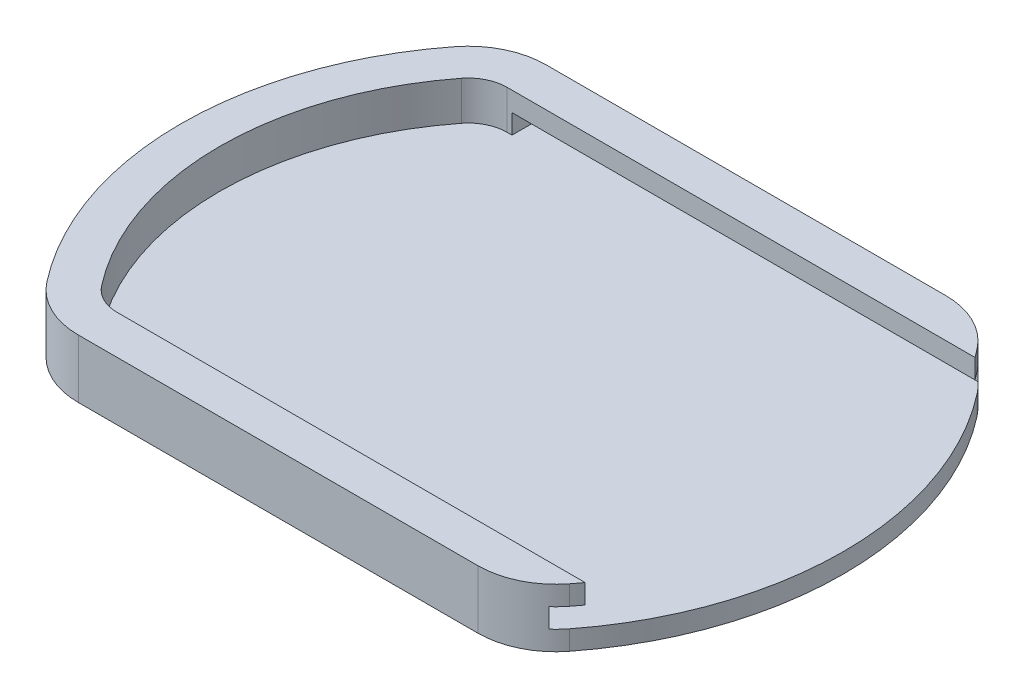
ISO-10303-21;
HEADER;
FILE_DESCRIPTION(('STEP AP214'),'2;1');
FILE_NAME('part.step','',(''),(''),'','','');
FILE_SCHEMA(('AUTOMOTIVE_DESIGN { 1 0 10303 214 1 1 1 1 }'));
ENDSEC;
DATA;
#1=APPLICATION_CONTEXT('core data for automotive mechanical design processes');
#2=APPLICATION_PROTOCOL_DEFINITION('international standard','automotive_design',2000,#1);
#3=PRODUCT_CONTEXT('',#1,'mechanical');
#4=PRODUCT('Part','Part','',(#3));
#5=PRODUCT_RELATED_PRODUCT_CATEGORY('part','',(#4));
#6=PRODUCT_DEFINITION_FORMATION('','',#4);
#7=PRODUCT_DEFINITION_CONTEXT('part definition',#1,'design');
#8=PRODUCT_DEFINITION('design','',#6,#7);
#9=PRODUCT_DEFINITION_SHAPE('','',#8);
#10=(LENGTH_UNIT() NAMED_UNIT(*) SI_UNIT(.MILLI.,.METRE.));
#11=(NAMED_UNIT(*) PLANE_ANGLE_UNIT() SI_UNIT($,.RADIAN.));
#12=(NAMED_UNIT(*) SI_UNIT($,.STERADIAN.) SOLID_ANGLE_UNIT());
#13=UNCERTAINTY_MEASURE_WITH_UNIT(LENGTH_MEASURE(1.E-05),#10,'distance_accuracy_value','');
#14=(GEOMETRIC_REPRESENTATION_CONTEXT(3) GLOBAL_UNCERTAINTY_ASSIGNED_CONTEXT((#13)) GLOBAL_UNIT_ASSIGNED_CONTEXT((#10,
#11,#12)) REPRESENTATION_CONTEXT('',''));
#15=CARTESIAN_POINT('',(0.,0.,0.));
#16=DIRECTION('',(0.,0.,1.));
#17=DIRECTION('',(1.,0.,0.));
#18=AXIS2_PLACEMENT_3D('',#15,#16,#17);
#19=CARTESIAN_POINT('',(0.,1.,0.));
#20=DIRECTION('',(0.,-1.,0.));
#21=DIRECTION('',(0.,0.,-1.));
#22=AXIS2_PLACEMENT_3D('',#19,#20,#21);
#23=CYLINDRICAL_SURFACE('',#22,17.);
#24=CARTESIAN_POINT('',(0.,2.,0.));
#25=DIRECTION('',(0.,1.,0.));
#26=DIRECTION('',(0.,0.,1.));
#27=AXIS2_PLACEMENT_3D('',#24,#25,#26);
#28=CIRCLE('',#27,17.);
#29=CARTESIAN_POINT('',(13.3998586939472,2.,-10.4615384615385));
#30=VERTEX_POINT('',#29);
#31=CARTESIAN_POINT('',(13.7477270848675,2.,-10.));
#32=VERTEX_POINT('',#31);
#33=EDGE_CURVE('E415',#30,#32,#28,.F.);
#34=ORIENTED_EDGE('',*,*,#33,.F.);
#35=DIRECTION('',(0.,-1.,0.));
#36=VECTOR('',#35,1.);
#37=CARTESIAN_POINT('',(13.3998586939472,1.,-10.4615384615385));
#38=LINE('',#37,#36);
#39=CARTESIAN_POINT('',(13.3998586939472,3.,-10.4615384615385));
#40=VERTEX_POINT('',#39);
#41=EDGE_CURVE('E283',#40,#30,#38,.T.);
#42=ORIENTED_EDGE('',*,*,#41,.F.);
#43=CARTESIAN_POINT('',(0.,3.,0.));
#44=DIRECTION('',(0.,1.,0.));
#45=DIRECTION('',(0.,0.,1.));
#46=AXIS2_PLACEMENT_3D('',#43,#44,#45);
#47=CIRCLE('',#46,17.);
#48=CARTESIAN_POINT('',(13.7477270848675,3.,-10.));
#49=VERTEX_POINT('',#48);
#50=EDGE_CURVE('E318',#49,#40,#47,.T.);
#51=ORIENTED_EDGE('',*,*,#50,.F.);
#52=DIRECTION('',(0.,-1.,0.));
#53=VECTOR('',#52,1.);
#54=CARTESIAN_POINT('',(13.7477270848675,3.,-10.));
#55=LINE('',#54,#53);
#56=EDGE_CURVE('E235',#49,#32,#55,.T.);
#57=ORIENTED_EDGE('',*,*,#56,.T.);
#58=EDGE_LOOP('',(#34,#42,#51,#57));
#59=FACE_BOUND('',#58,.T.);
#60=ADVANCED_FACE('F41',(#59),#23,.T.);
#61=CARTESIAN_POINT('',(13.3998586939472,1.,-10.4615384615385));
#62=VERTEX_POINT('',#61);
#63=CARTESIAN_POINT('',(13.3998586939472,0.,-10.4615384615385));
#64=VERTEX_POINT('',#63);
#65=EDGE_CURVE('E281',#62,#64,#38,.T.);
#66=ORIENTED_EDGE('',*,*,#65,.F.);
#67=CARTESIAN_POINT('',(0.,1.,0.));
#68=DIRECTION('',(0.,1.,0.));
#69=DIRECTION('',(0.,0.,1.));
#70=AXIS2_PLACEMENT_3D('',#67,#68,#69);
#71=CIRCLE('',#70,17.);
#72=CARTESIAN_POINT('',(13.3998586939472,1.,10.4615384615385));
#73=VERTEX_POINT('',#72);
#74=EDGE_CURVE('E245',#62,#73,#71,.F.);
#75=ORIENTED_EDGE('',*,*,#74,.T.);
#76=DIRECTION('',(0.,-1.,0.));
#77=VECTOR('',#76,1.);
#78=CARTESIAN_POINT('',(13.3998586939472,1.,10.4615384615385));
#79=LINE('',#78,#77);
#80=CARTESIAN_POINT('',(13.3998586939472,0.,10.4615384615385));
#81=VERTEX_POINT('',#80);
#82=EDGE_CURVE('E243',#73,#81,#79,.T.);
#83=ORIENTED_EDGE('',*,*,#82,.T.);
#84=CARTESIAN_POINT('',(0.,0.,0.));
#85=DIRECTION('',(0.,1.,0.));
#86=DIRECTION('',(0.,0.,1.));
#87=AXIS2_PLACEMENT_3D('',#84,#85,#86);
#88=CIRCLE('',#87,17.);
#89=EDGE_CURVE('E244',#64,#81,#88,.F.);
#90=ORIENTED_EDGE('',*,*,#89,.F.);
#91=EDGE_LOOP('',(#66,#75,#83,#90));
#92=FACE_BOUND('',#91,.T.);
#93=ADVANCED_FACE('F441',(#92),#23,.T.);
#94=CARTESIAN_POINT('',(0.,1.,0.));
#95=DIRECTION('',(0.,1.,0.));
#96=DIRECTION('',(0.,0.,1.));
#97=AXIS2_PLACEMENT_3D('',#94,#95,#96);
#98=PLANE('',#97);
#99=CARTESIAN_POINT('',(-10.2469507659596,1.,8.));
#100=DIRECTION('',(0.,1.,0.));
#101=DIRECTION('',(0.,0.,1.));
#102=AXIS2_PLACEMENT_3D('',#99,#100,#101);
#103=CIRCLE('',#102,2.);
#104=CARTESIAN_POINT('',(-11.8234047299534,1.,9.23076923076923));
#105=VERTEX_POINT('',#104);
#106=CARTESIAN_POINT('',(-10.2469507659596,1.,10.));
#107=VERTEX_POINT('',#106);
#108=EDGE_CURVE('E218',#105,#107,#103,.T.);
#109=ORIENTED_EDGE('',*,*,#108,.T.);
#110=DIRECTION('',(1.,0.,0.));
#111=VECTOR('',#110,1.);
#112=CARTESIAN_POINT('',(0.,1.,10.));
#113=LINE('',#112,#111);
#114=CARTESIAN_POINT('',(-10.,1.,10.));
#115=VERTEX_POINT('',#114);
#116=EDGE_CURVE('E214',#107,#115,#113,.T.);
#117=ORIENTED_EDGE('',*,*,#116,.T.);
#118=DIRECTION('',(0.,0.,-1.));
#119=VECTOR('',#118,1.);
#120=CARTESIAN_POINT('',(-10.,1.,10.));
#121=LINE('',#120,#119);
#122=CARTESIAN_POINT('',(-10.,1.,11.));
#123=VERTEX_POINT('',#122);
#124=EDGE_CURVE('E61',#123,#115,#121,.T.);
#125=ORIENTED_EDGE('',*,*,#124,.F.);
#126=DIRECTION('',(1.,0.,0.));
#127=VECTOR('',#126,1.);
#128=CARTESIAN_POINT('',(-10.,1.,11.));
#129=LINE('',#128,#127);
#130=CARTESIAN_POINT('',(12.8927020770242,1.,11.));
#131=VERTEX_POINT('',#130);
#132=EDGE_CURVE('E291',#123,#131,#129,.T.);
#133=ORIENTED_EDGE('',*,*,#132,.T.);
#134=CARTESIAN_POINT('',(10.2469507659596,1.,8.));
#135=DIRECTION('',(0.,-1.,0.));
#136=DIRECTION('',(0.,0.,-1.));
#137=AXIS2_PLACEMENT_3D('',#134,#135,#136);
#138=CIRCLE('',#137,4.);
#139=EDGE_CURVE('E296',#131,#73,#138,.F.);
#140=ORIENTED_EDGE('',*,*,#139,.T.);
#141=ORIENTED_EDGE('',*,*,#74,.F.);
#142=CARTESIAN_POINT('',(10.2469507659596,1.,-8.));
#143=DIRECTION('',(0.,-1.,0.));
#144=DIRECTION('',(0.,0.,-1.));
#145=AXIS2_PLACEMENT_3D('',#142,#143,#144);
#146=CIRCLE('',#145,4.);
#147=CARTESIAN_POINT('',(12.8927020770242,1.,-11.));
#148=VERTEX_POINT('',#147);
#149=EDGE_CURVE('E420',#148,#62,#146,.T.);
#150=ORIENTED_EDGE('',*,*,#149,.F.);
#151=DIRECTION('',(1.,0.,0.));
#152=VECTOR('',#151,1.);
#153=CARTESIAN_POINT('',(-10.,1.,-11.));
#154=LINE('',#153,#152);
#155=CARTESIAN_POINT('',(-10.,1.,-11.));
#156=VERTEX_POINT('',#155);
#157=EDGE_CURVE('E203',#156,#148,#154,.T.);
#158=ORIENTED_EDGE('',*,*,#157,.F.);
#159=DIRECTION('',(0.,0.,-1.));
#160=VECTOR('',#159,1.);
#161=CARTESIAN_POINT('',(-10.,1.,-10.));
#162=LINE('',#161,#160);
#163=CARTESIAN_POINT('',(-10.,1.,-10.));
#164=VERTEX_POINT('',#163);
#165=EDGE_CURVE('E194',#164,#156,#162,.T.);
#166=ORIENTED_EDGE('',*,*,#165,.F.);
#167=DIRECTION('',(-1.,0.,0.));
#168=VECTOR('',#167,1.);
#169=CARTESIAN_POINT('',(0.,1.,-10.));
#170=LINE('',#169,#168);
#171=CARTESIAN_POINT('',(-10.2469507659596,1.,-10.));
#172=VERTEX_POINT('',#171);
#173=EDGE_CURVE('E196',#164,#172,#170,.T.);
#174=ORIENTED_EDGE('',*,*,#173,.T.);
#175=CARTESIAN_POINT('',(-10.2469507659596,1.,-8.));
#176=DIRECTION('',(0.,1.,0.));
#177=DIRECTION('',(0.,0.,1.));
#178=AXIS2_PLACEMENT_3D('',#175,#176,#177);
#179=CIRCLE('',#178,2.);
#180=CARTESIAN_POINT('',(-11.8234047299534,1.,-9.23076923076924));
#181=VERTEX_POINT('',#180);
#182=EDGE_CURVE('E216',#172,#181,#179,.T.);
#183=ORIENTED_EDGE('',*,*,#182,.T.);
#184=CARTESIAN_POINT('',(0.,1.,0.));
#185=DIRECTION('',(0.,1.,0.));
#186=DIRECTION('',(0.,0.,1.));
#187=AXIS2_PLACEMENT_3D('',#184,#185,#186);
#188=CIRCLE('',#187,15.);
#189=EDGE_CURVE('E222',#181,#105,#188,.T.);
#190=ORIENTED_EDGE('',*,*,#189,.T.);
#191=EDGE_LOOP('',(#109,#117,#125,#133,#140,#141,#150,#158,#166,#174,#183,#190));
#192=FACE_BOUND('',#191,.T.);
#193=ADVANCED_FACE('F195',(#192),#98,.T.);
#194=CARTESIAN_POINT('',(0.,2.,0.));
#195=DIRECTION('',(0.,1.,0.));
#196=DIRECTION('',(0.,0.,1.));
#197=AXIS2_PLACEMENT_3D('',#194,#195,#196);
#198=CIRCLE('',#197,17.);
#199=CARTESIAN_POINT('',(13.7477270848675,2.,10.));
#200=VERTEX_POINT('',#199);
#201=CARTESIAN_POINT('',(13.3998586939472,2.,10.4615384615385));
#202=VERTEX_POINT('',#201);
#203=EDGE_CURVE('E305',#200,#202,#198,.F.);
#204=ORIENTED_EDGE('',*,*,#203,.F.);
#205=DIRECTION('',(0.,-1.,0.));
#206=VECTOR('',#205,1.);
#207=CARTESIAN_POINT('',(13.7477270848675,3.,10.));
#208=LINE('',#207,#206);
#209=CARTESIAN_POINT('',(13.7477270848675,3.,10.));
#210=VERTEX_POINT('',#209);
#211=EDGE_CURVE('E232',#210,#200,#208,.T.);
#212=ORIENTED_EDGE('',*,*,#211,.F.);
#213=CARTESIAN_POINT('',(13.3998586939472,3.,10.4615384615385));
#214=VERTEX_POINT('',#213);
#215=EDGE_CURVE('E325',#214,#210,#47,.T.);
#216=ORIENTED_EDGE('',*,*,#215,.F.);
#217=EDGE_CURVE('E270',#214,#202,#79,.T.);
#218=ORIENTED_EDGE('',*,*,#217,.T.);
#219=EDGE_LOOP('',(#204,#212,#216,#218));
#220=FACE_BOUND('',#219,.T.);
#221=ADVANCED_FACE('F43',(#220),#23,.T.);
#222=CARTESIAN_POINT('',(10.2469507659596,1.,-8.));
#223=DIRECTION('',(0.,-1.,0.));
#224=DIRECTION('',(0.,0.,-1.));
#225=AXIS2_PLACEMENT_3D('',#222,#223,#224);
#226=CYLINDRICAL_SURFACE('',#225,4.);
#227=ORIENTED_EDGE('',*,*,#41,.T.);
#228=CARTESIAN_POINT('',(10.2469507659596,2.,-8.));
#229=DIRECTION('',(0.,1.,0.));
#230=DIRECTION('',(0.,0.,1.));
#231=AXIS2_PLACEMENT_3D('',#228,#229,#230);
#232=CIRCLE('',#231,4.);
#233=CARTESIAN_POINT('',(12.8927020770242,2.,-11.));
#234=VERTEX_POINT('',#233);
#235=EDGE_CURVE('E417',#30,#234,#232,.T.);
#236=ORIENTED_EDGE('',*,*,#235,.T.);
#237=DIRECTION('',(0.,-1.,0.));
#238=VECTOR('',#237,1.);
#239=CARTESIAN_POINT('',(12.8927020770242,1.,-11.));
#240=LINE('',#239,#238);
#241=EDGE_CURVE('E11',#234,#148,#240,.T.);
#242=ORIENTED_EDGE('',*,*,#241,.T.);
#243=ORIENTED_EDGE('',*,*,#149,.T.);
#244=ORIENTED_EDGE('',*,*,#65,.T.);
#245=CARTESIAN_POINT('',(10.2469507659596,0.,-8.));
#246=DIRECTION('',(0.,1.,0.));
#247=DIRECTION('',(0.,0.,1.));
#248=AXIS2_PLACEMENT_3D('',#245,#246,#247);
#249=CIRCLE('',#248,4.);
#250=CARTESIAN_POINT('',(10.2469507659596,0.,-12.));
#251=VERTEX_POINT('',#250);
#252=EDGE_CURVE('E248',#64,#251,#249,.T.);
#253=ORIENTED_EDGE('',*,*,#252,.T.);
#254=DIRECTION('',(0.,-1.,0.));
#255=VECTOR('',#254,1.);
#256=CARTESIAN_POINT('',(10.2469507659596,1.,-12.));
#257=LINE('',#256,#255);
#258=CARTESIAN_POINT('',(10.2469507659596,3.,-12.));
#259=VERTEX_POINT('',#258);
#260=EDGE_CURVE('E284',#259,#251,#257,.T.);
#261=ORIENTED_EDGE('',*,*,#260,.F.);
#262=CARTESIAN_POINT('',(10.2469507659596,3.,-8.));
#263=DIRECTION('',(0.,1.,0.));
#264=DIRECTION('',(0.,0.,1.));
#265=AXIS2_PLACEMENT_3D('',#262,#263,#264);
#266=CIRCLE('',#265,4.);
#267=EDGE_CURVE('E321',#40,#259,#266,.T.);
#268=ORIENTED_EDGE('',*,*,#267,.F.);
#269=EDGE_LOOP('',(#227,#236,#242,#243,#244,#253,#261,#268));
#270=FACE_BOUND('',#269,.T.);
#271=ADVANCED_FACE('F374',(#270),#226,.T.);
#272=CARTESIAN_POINT('',(0.,1.,-12.));
#273=DIRECTION('',(0.,0.,-1.));
#274=DIRECTION('',(-1.,0.,0.));
#275=AXIS2_PLACEMENT_3D('',#272,#273,#274);
#276=PLANE('',#275);
#277=DIRECTION('',(1.,0.,0.));
#278=VECTOR('',#277,1.);
#279=CARTESIAN_POINT('',(0.,0.,-12.));
#280=LINE('',#279,#278);
#281=CARTESIAN_POINT('',(-10.2469507659596,0.,-12.));
#282=VERTEX_POINT('',#281);
#283=EDGE_CURVE('E252',#282,#251,#280,.T.);
#284=ORIENTED_EDGE('',*,*,#283,.F.);
#285=DIRECTION('',(0.,-1.,0.));
#286=VECTOR('',#285,1.);
#287=CARTESIAN_POINT('',(-10.2469507659596,1.,-12.));
#288=LINE('',#287,#286);
#289=CARTESIAN_POINT('',(-10.2469507659596,3.,-12.));
#290=VERTEX_POINT('',#289);
#291=EDGE_CURVE('E278',#290,#282,#288,.T.);
#292=ORIENTED_EDGE('',*,*,#291,.F.);
#293=DIRECTION('',(-1.,0.,0.));
#294=VECTOR('',#293,1.);
#295=CARTESIAN_POINT('',(0.,3.,-12.));
#296=LINE('',#295,#294);
#297=EDGE_CURVE('E324',#259,#290,#296,.T.);
#298=ORIENTED_EDGE('',*,*,#297,.F.);
#299=ORIENTED_EDGE('',*,*,#260,.T.);
#300=EDGE_LOOP('',(#284,#292,#298,#299));
#301=FACE_BOUND('',#300,.T.);
#302=ADVANCED_FACE('F379',(#301),#276,.T.);
#303=CARTESIAN_POINT('',(-10.2469507659596,1.,-8.));
#304=DIRECTION('',(0.,-1.,0.));
#305=DIRECTION('',(0.,0.,-1.));
#306=AXIS2_PLACEMENT_3D('',#303,#304,#305);
#307=CYLINDRICAL_SURFACE('',#306,4.);
#308=CARTESIAN_POINT('',(-10.2469507659596,0.,-8.));
#309=DIRECTION('',(0.,1.,0.));
#310=DIRECTION('',(0.,0.,1.));
#311=AXIS2_PLACEMENT_3D('',#308,#309,#310);
#312=CIRCLE('',#311,4.);
#313=CARTESIAN_POINT('',(-13.3998586939472,0.,-10.4615384615385));
#314=VERTEX_POINT('',#313);
#315=EDGE_CURVE('E254',#314,#282,#312,.F.);
#316=ORIENTED_EDGE('',*,*,#315,.F.);
#317=DIRECTION('',(0.,-1.,0.));
#318=VECTOR('',#317,1.);
#319=CARTESIAN_POINT('',(-13.3998586939472,1.,-10.4615384615385));
#320=LINE('',#319,#318);
#321=CARTESIAN_POINT('',(-13.3998586939472,3.,-10.4615384615385));
#322=VERTEX_POINT('',#321);
#323=EDGE_CURVE('E279',#322,#314,#320,.T.);
#324=ORIENTED_EDGE('',*,*,#323,.F.);
#325=CARTESIAN_POINT('',(-10.2469507659596,3.,-8.));
#326=DIRECTION('',(0.,1.,0.));
#327=DIRECTION('',(0.,0.,1.));
#328=AXIS2_PLACEMENT_3D('',#325,#326,#327);
#329=CIRCLE('',#328,4.);
#330=EDGE_CURVE('E327',#290,#322,#329,.T.);
#331=ORIENTED_EDGE('',*,*,#330,.F.);
#332=ORIENTED_EDGE('',*,*,#291,.T.);
#333=EDGE_LOOP('',(#316,#324,#331,#332));
#334=FACE_BOUND('',#333,.T.);
#335=ADVANCED_FACE('F384',(#334),#307,.T.);
#336=CARTESIAN_POINT('',(0.,1.,0.));
#337=DIRECTION('',(0.,-1.,0.));
#338=DIRECTION('',(0.,0.,-1.));
#339=AXIS2_PLACEMENT_3D('',#336,#337,#338);
#340=CYLINDRICAL_SURFACE('',#339,17.);
#341=CARTESIAN_POINT('',(0.,0.,0.));
#342=DIRECTION('',(0.,1.,0.));
#343=DIRECTION('',(0.,0.,1.));
#344=AXIS2_PLACEMENT_3D('',#341,#342,#343);
#345=CIRCLE('',#344,17.);
#346=CARTESIAN_POINT('',(-13.3998586939472,0.,10.4615384615385));
#347=VERTEX_POINT('',#346);
#348=EDGE_CURVE('E256',#314,#347,#345,.T.);
#349=ORIENTED_EDGE('',*,*,#348,.T.);
#350=DIRECTION('',(0.,-1.,0.));
#351=VECTOR('',#350,1.);
#352=CARTESIAN_POINT('',(-13.3998586939472,1.,10.4615384615385));
#353=LINE('',#352,#351);
#354=CARTESIAN_POINT('',(-13.3998586939472,3.,10.4615384615385));
#355=VERTEX_POINT('',#354);
#356=EDGE_CURVE('E274',#355,#347,#353,.T.);
#357=ORIENTED_EDGE('',*,*,#356,.F.);
#358=CARTESIAN_POINT('',(0.,3.,0.));
#359=DIRECTION('',(0.,1.,0.));
#360=DIRECTION('',(0.,0.,1.));
#361=AXIS2_PLACEMENT_3D('',#358,#359,#360);
#362=CIRCLE('',#361,17.);
#363=EDGE_CURVE('E332',#322,#355,#362,.T.);
#364=ORIENTED_EDGE('',*,*,#363,.F.);
#365=ORIENTED_EDGE('',*,*,#323,.T.);
#366=EDGE_LOOP('',(#349,#357,#364,#365));
#367=FACE_BOUND('',#366,.T.);
#368=ADVANCED_FACE('F389',(#367),#340,.T.);
#369=CARTESIAN_POINT('',(-10.2469507659596,1.,8.));
#370=DIRECTION('',(0.,-1.,0.));
#371=DIRECTION('',(0.,0.,-1.));
#372=AXIS2_PLACEMENT_3D('',#369,#370,#371);
#373=CYLINDRICAL_SURFACE('',#372,4.);
#374=CARTESIAN_POINT('',(-10.2469507659596,0.,8.));
#375=DIRECTION('',(0.,1.,0.));
#376=DIRECTION('',(0.,0.,1.));
#377=AXIS2_PLACEMENT_3D('',#374,#375,#376);
#378=CIRCLE('',#377,4.);
#379=CARTESIAN_POINT('',(-10.2469507659596,0.,12.));
#380=VERTEX_POINT('',#379);
#381=EDGE_CURVE('E257',#347,#380,#378,.T.);
#382=ORIENTED_EDGE('',*,*,#381,.T.);
#383=DIRECTION('',(0.,-1.,0.));
#384=VECTOR('',#383,1.);
#385=CARTESIAN_POINT('',(-10.2469507659596,1.,12.));
#386=LINE('',#385,#384);
#387=CARTESIAN_POINT('',(-10.2469507659596,3.,12.));
#388=VERTEX_POINT('',#387);
#389=EDGE_CURVE('E275',#388,#380,#386,.T.);
#390=ORIENTED_EDGE('',*,*,#389,.F.);
#391=CARTESIAN_POINT('',(-10.2469507659596,3.,8.));
#392=DIRECTION('',(0.,1.,0.));
#393=DIRECTION('',(0.,0.,1.));
#394=AXIS2_PLACEMENT_3D('',#391,#392,#393);
#395=CIRCLE('',#394,4.);
#396=EDGE_CURVE('E331',#355,#388,#395,.T.);
#397=ORIENTED_EDGE('',*,*,#396,.F.);
#398=ORIENTED_EDGE('',*,*,#356,.T.);
#399=EDGE_LOOP('',(#382,#390,#397,#398));
#400=FACE_BOUND('',#399,.T.);
#401=ADVANCED_FACE('F391',(#400),#373,.T.);
#402=CARTESIAN_POINT('',(0.,1.,12.));
#403=DIRECTION('',(0.,0.,-1.));
#404=DIRECTION('',(-1.,0.,0.));
#405=AXIS2_PLACEMENT_3D('',#402,#403,#404);
#406=PLANE('',#405);
#407=DIRECTION('',(1.,0.,0.));
#408=VECTOR('',#407,1.);
#409=CARTESIAN_POINT('',(0.,0.,12.));
#410=LINE('',#409,#408);
#411=CARTESIAN_POINT('',(10.2469507659596,0.,12.));
#412=VERTEX_POINT('',#411);
#413=EDGE_CURVE('E265',#380,#412,#410,.T.);
#414=ORIENTED_EDGE('',*,*,#413,.T.);
#415=DIRECTION('',(0.,-1.,0.));
#416=VECTOR('',#415,1.);
#417=CARTESIAN_POINT('',(10.2469507659596,1.,12.));
#418=LINE('',#417,#416);
#419=CARTESIAN_POINT('',(10.2469507659596,3.,12.));
#420=VERTEX_POINT('',#419);
#421=EDGE_CURVE('E269',#420,#412,#418,.T.);
#422=ORIENTED_EDGE('',*,*,#421,.F.);
#423=DIRECTION('',(1.,0.,0.));
#424=VECTOR('',#423,1.);
#425=CARTESIAN_POINT('',(0.,3.,12.));
#426=LINE('',#425,#424);
#427=EDGE_CURVE('E339',#388,#420,#426,.T.);
#428=ORIENTED_EDGE('',*,*,#427,.F.);
#429=ORIENTED_EDGE('',*,*,#389,.T.);
#430=EDGE_LOOP('',(#414,#422,#428,#429));
#431=FACE_BOUND('',#430,.T.);
#432=ADVANCED_FACE('F399',(#431),#406,.F.);
#433=CARTESIAN_POINT('',(10.2469507659596,1.,8.));
#434=DIRECTION('',(0.,-1.,0.));
#435=DIRECTION('',(0.,0.,-1.));
#436=AXIS2_PLACEMENT_3D('',#433,#434,#435);
#437=CYLINDRICAL_SURFACE('',#436,4.);
#438=ORIENTED_EDGE('',*,*,#139,.F.);
#439=DIRECTION('',(0.,-1.,0.));
#440=VECTOR('',#439,1.);
#441=CARTESIAN_POINT('',(12.8927020770242,1.,11.));
#442=LINE('',#441,#440);
#443=CARTESIAN_POINT('',(12.8927020770242,2.,11.));
#444=VERTEX_POINT('',#443);
#445=EDGE_CURVE('E47',#444,#131,#442,.T.);
#446=ORIENTED_EDGE('',*,*,#445,.F.);
#447=CARTESIAN_POINT('',(10.2469507659596,2.,8.));
#448=DIRECTION('',(0.,1.,0.));
#449=DIRECTION('',(0.,0.,1.));
#450=AXIS2_PLACEMENT_3D('',#447,#448,#449);
#451=CIRCLE('',#450,4.);
#452=EDGE_CURVE('E301',#202,#444,#451,.F.);
#453=ORIENTED_EDGE('',*,*,#452,.F.);
#454=ORIENTED_EDGE('',*,*,#217,.F.);
#455=CARTESIAN_POINT('',(10.2469507659596,3.,8.));
#456=DIRECTION('',(0.,1.,0.));
#457=DIRECTION('',(0.,0.,1.));
#458=AXIS2_PLACEMENT_3D('',#455,#456,#457);
#459=CIRCLE('',#458,4.);
#460=EDGE_CURVE('E338',#420,#214,#459,.T.);
#461=ORIENTED_EDGE('',*,*,#460,.F.);
#462=ORIENTED_EDGE('',*,*,#421,.T.);
#463=CARTESIAN_POINT('',(10.2469507659596,0.,8.));
#464=DIRECTION('',(0.,1.,0.));
#465=DIRECTION('',(0.,0.,1.));
#466=AXIS2_PLACEMENT_3D('',#463,#464,#465);
#467=CIRCLE('',#466,4.);
#468=EDGE_CURVE('E246',#81,#412,#467,.F.);
#469=ORIENTED_EDGE('',*,*,#468,.F.);
#470=ORIENTED_EDGE('',*,*,#82,.F.);
#471=EDGE_LOOP('',(#438,#446,#453,#454,#461,#462,#469,#470));
#472=FACE_BOUND('',#471,.T.);
#473=ADVANCED_FACE('F304',(#472),#437,.T.);
#474=CARTESIAN_POINT('',(0.,0.,0.));
#475=DIRECTION('',(0.,1.,0.));
#476=DIRECTION('',(0.,0.,1.));
#477=AXIS2_PLACEMENT_3D('',#474,#475,#476);
#478=PLANE('',#477);
#479=ORIENTED_EDGE('',*,*,#89,.T.);
#480=ORIENTED_EDGE('',*,*,#468,.T.);
#481=ORIENTED_EDGE('',*,*,#413,.F.);
#482=ORIENTED_EDGE('',*,*,#381,.F.);
#483=ORIENTED_EDGE('',*,*,#348,.F.);
#484=ORIENTED_EDGE('',*,*,#315,.T.);
#485=ORIENTED_EDGE('',*,*,#283,.T.);
#486=ORIENTED_EDGE('',*,*,#252,.F.);
#487=EDGE_LOOP('',(#479,#480,#481,#482,#483,#484,#485,#486));
#488=FACE_BOUND('',#487,.T.);
#489=ADVANCED_FACE('F392',(#488),#478,.F.);
#490=CARTESIAN_POINT('',(0.,3.,0.));
#491=DIRECTION('',(0.,-1.,0.));
#492=DIRECTION('',(0.,0.,-1.));
#493=AXIS2_PLACEMENT_3D('',#490,#491,#492);
#494=CYLINDRICAL_SURFACE('',#493,15.);
#495=ORIENTED_EDGE('',*,*,#189,.F.);
#496=DIRECTION('',(0.,-1.,0.));
#497=VECTOR('',#496,1.);
#498=CARTESIAN_POINT('',(-11.8234047299534,3.,-9.23076923076924));
#499=LINE('',#498,#497);
#500=CARTESIAN_POINT('',(-11.8234047299534,3.,-9.23076923076924));
#501=VERTEX_POINT('',#500);
#502=EDGE_CURVE('E239',#501,#181,#499,.T.);
#503=ORIENTED_EDGE('',*,*,#502,.F.);
#504=CARTESIAN_POINT('',(0.,3.,0.));
#505=DIRECTION('',(0.,1.,0.));
#506=DIRECTION('',(0.,0.,1.));
#507=AXIS2_PLACEMENT_3D('',#504,#505,#506);
#508=CIRCLE('',#507,15.);
#509=CARTESIAN_POINT('',(-11.8234047299534,3.,9.23076923076923));
#510=VERTEX_POINT('',#509);
#511=EDGE_CURVE('E227',#501,#510,#508,.T.);
#512=ORIENTED_EDGE('',*,*,#511,.T.);
#513=DIRECTION('',(0.,-1.,0.));
#514=VECTOR('',#513,1.);
#515=CARTESIAN_POINT('',(-11.8234047299534,3.,9.23076923076923));
#516=LINE('',#515,#514);
#517=EDGE_CURVE('E229',#510,#105,#516,.T.);
#518=ORIENTED_EDGE('',*,*,#517,.T.);
#519=EDGE_LOOP('',(#495,#503,#512,#518));
#520=FACE_BOUND('',#519,.T.);
#521=ADVANCED_FACE('F365',(#520),#494,.F.);
#522=CARTESIAN_POINT('',(-10.2469507659596,3.,-8.));
#523=DIRECTION('',(0.,-1.,0.));
#524=DIRECTION('',(0.,0.,-1.));
#525=AXIS2_PLACEMENT_3D('',#522,#523,#524);
#526=CYLINDRICAL_SURFACE('',#525,2.);
#527=ORIENTED_EDGE('',*,*,#182,.F.);
#528=DIRECTION('',(0.,-1.,0.));
#529=VECTOR('',#528,1.);
#530=CARTESIAN_POINT('',(-10.2469507659596,3.,-10.));
#531=LINE('',#530,#529);
#532=CARTESIAN_POINT('',(-10.2469507659596,3.,-10.));
#533=VERTEX_POINT('',#532);
#534=EDGE_CURVE('E213',#533,#172,#531,.T.);
#535=ORIENTED_EDGE('',*,*,#534,.F.);
#536=CARTESIAN_POINT('',(-10.2469507659596,3.,-8.));
#537=DIRECTION('',(0.,1.,0.));
#538=DIRECTION('',(0.,0.,1.));
#539=AXIS2_PLACEMENT_3D('',#536,#537,#538);
#540=CIRCLE('',#539,2.);
#541=EDGE_CURVE('E311',#533,#501,#540,.T.);
#542=ORIENTED_EDGE('',*,*,#541,.T.);
#543=ORIENTED_EDGE('',*,*,#502,.T.);
#544=EDGE_LOOP('',(#527,#535,#542,#543));
#545=FACE_BOUND('',#544,.T.);
#546=ADVANCED_FACE('F368',(#545),#526,.F.);
#547=CARTESIAN_POINT('',(0.,3.,-10.));
#548=DIRECTION('',(0.,0.,1.));
#549=DIRECTION('',(1.,0.,0.));
#550=AXIS2_PLACEMENT_3D('',#547,#548,#549);
#551=PLANE('',#550);
#552=DIRECTION('',(1.,0.,0.));
#553=VECTOR('',#552,1.);
#554=CARTESIAN_POINT('',(-10.,2.,-10.));
#555=LINE('',#554,#553);
#556=CARTESIAN_POINT('',(-10.,2.,-10.));
#557=VERTEX_POINT('',#556);
#558=EDGE_CURVE('E369',#557,#32,#555,.T.);
#559=ORIENTED_EDGE('',*,*,#558,.T.);
#560=ORIENTED_EDGE('',*,*,#56,.F.);
#561=DIRECTION('',(-1.,0.,0.));
#562=VECTOR('',#561,1.);
#563=CARTESIAN_POINT('',(0.,3.,-10.));
#564=LINE('',#563,#562);
#565=EDGE_CURVE('E316',#49,#533,#564,.T.);
#566=ORIENTED_EDGE('',*,*,#565,.T.);
#567=ORIENTED_EDGE('',*,*,#534,.T.);
#568=ORIENTED_EDGE('',*,*,#173,.F.);
#569=DIRECTION('',(0.,-1.,0.));
#570=VECTOR('',#569,1.);
#571=CARTESIAN_POINT('',(-10.,1.,-10.));
#572=LINE('',#571,#570);
#573=EDGE_CURVE('E204',#557,#164,#572,.T.);
#574=ORIENTED_EDGE('',*,*,#573,.F.);
#575=EDGE_LOOP('',(#559,#560,#566,#567,#568,#574));
#576=FACE_BOUND('',#575,.T.);
#577=ADVANCED_FACE('F211',(#576),#551,.T.);
#578=CARTESIAN_POINT('',(0.,3.,10.));
#579=DIRECTION('',(0.,0.,-1.));
#580=DIRECTION('',(-1.,0.,0.));
#581=AXIS2_PLACEMENT_3D('',#578,#579,#580);
#582=PLANE('',#581);
#583=DIRECTION('',(1.,0.,0.));
#584=VECTOR('',#583,1.);
#585=CARTESIAN_POINT('',(-10.,2.,10.));
#586=LINE('',#585,#584);
#587=CARTESIAN_POINT('',(-10.,2.,10.));
#588=VERTEX_POINT('',#587);
#589=EDGE_CURVE('E404',#588,#200,#586,.T.);
#590=ORIENTED_EDGE('',*,*,#589,.F.);
#591=DIRECTION('',(0.,1.,0.));
#592=VECTOR('',#591,1.);
#593=CARTESIAN_POINT('',(-10.,2.,10.));
#594=LINE('',#593,#592);
#595=EDGE_CURVE('E362',#115,#588,#594,.T.);
#596=ORIENTED_EDGE('',*,*,#595,.F.);
#597=ORIENTED_EDGE('',*,*,#116,.F.);
#598=DIRECTION('',(0.,-1.,0.));
#599=VECTOR('',#598,1.);
#600=CARTESIAN_POINT('',(-10.2469507659596,3.,10.));
#601=LINE('',#600,#599);
#602=CARTESIAN_POINT('',(-10.2469507659596,3.,10.));
#603=VERTEX_POINT('',#602);
#604=EDGE_CURVE('E226',#603,#107,#601,.T.);
#605=ORIENTED_EDGE('',*,*,#604,.F.);
#606=DIRECTION('',(1.,0.,0.));
#607=VECTOR('',#606,1.);
#608=CARTESIAN_POINT('',(0.,3.,10.));
#609=LINE('',#608,#607);
#610=EDGE_CURVE('E344',#603,#210,#609,.T.);
#611=ORIENTED_EDGE('',*,*,#610,.T.);
#612=ORIENTED_EDGE('',*,*,#211,.T.);
#613=EDGE_LOOP('',(#590,#596,#597,#605,#611,#612));
#614=FACE_BOUND('',#613,.T.);
#615=ADVANCED_FACE('F363',(#614),#582,.T.);
#616=CARTESIAN_POINT('',(-10.2469507659596,3.,8.));
#617=DIRECTION('',(0.,-1.,0.));
#618=DIRECTION('',(0.,0.,-1.));
#619=AXIS2_PLACEMENT_3D('',#616,#617,#618);
#620=CYLINDRICAL_SURFACE('',#619,2.);
#621=ORIENTED_EDGE('',*,*,#108,.F.);
#622=ORIENTED_EDGE('',*,*,#517,.F.);
#623=CARTESIAN_POINT('',(-10.2469507659596,3.,8.));
#624=DIRECTION('',(0.,1.,0.));
#625=DIRECTION('',(0.,0.,1.));
#626=AXIS2_PLACEMENT_3D('',#623,#624,#625);
#627=CIRCLE('',#626,2.);
#628=EDGE_CURVE('E228',#510,#603,#627,.T.);
#629=ORIENTED_EDGE('',*,*,#628,.T.);
#630=ORIENTED_EDGE('',*,*,#604,.T.);
#631=EDGE_LOOP('',(#621,#622,#629,#630));
#632=FACE_BOUND('',#631,.T.);
#633=ADVANCED_FACE('F348',(#632),#620,.F.);
#634=CARTESIAN_POINT('',(0.,3.,0.));
#635=DIRECTION('',(0.,1.,0.));
#636=DIRECTION('',(0.,0.,1.));
#637=AXIS2_PLACEMENT_3D('',#634,#635,#636);
#638=PLANE('',#637);
#639=ORIENTED_EDGE('',*,*,#511,.F.);
#640=ORIENTED_EDGE('',*,*,#541,.F.);
#641=ORIENTED_EDGE('',*,*,#565,.F.);
#642=ORIENTED_EDGE('',*,*,#50,.T.);
#643=ORIENTED_EDGE('',*,*,#267,.T.);
#644=ORIENTED_EDGE('',*,*,#297,.T.);
#645=ORIENTED_EDGE('',*,*,#330,.T.);
#646=ORIENTED_EDGE('',*,*,#363,.T.);
#647=ORIENTED_EDGE('',*,*,#396,.T.);
#648=ORIENTED_EDGE('',*,*,#427,.T.);
#649=ORIENTED_EDGE('',*,*,#460,.T.);
#650=ORIENTED_EDGE('',*,*,#215,.T.);
#651=ORIENTED_EDGE('',*,*,#610,.F.);
#652=ORIENTED_EDGE('',*,*,#628,.F.);
#653=EDGE_LOOP('',(#639,#640,#641,#642,#643,#644,#645,#646,#647,#648,#649,#650,#651,#652));
#654=FACE_BOUND('',#653,.T.);
#655=ADVANCED_FACE('F353',(#654),#638,.T.);
#656=CARTESIAN_POINT('',(-10.,2.,11.));
#657=DIRECTION('',(0.,0.,1.));
#658=DIRECTION('',(1.,0.,0.));
#659=AXIS2_PLACEMENT_3D('',#656,#657,#658);
#660=PLANE('',#659);
#661=ORIENTED_EDGE('',*,*,#445,.T.);
#662=ORIENTED_EDGE('',*,*,#132,.F.);
#663=DIRECTION('',(0.,-1.,0.));
#664=VECTOR('',#663,1.);
#665=CARTESIAN_POINT('',(-10.,2.,11.));
#666=LINE('',#665,#664);
#667=CARTESIAN_POINT('',(-10.,2.,11.));
#668=VERTEX_POINT('',#667);
#669=EDGE_CURVE('E406',#668,#123,#666,.T.);
#670=ORIENTED_EDGE('',*,*,#669,.F.);
#671=DIRECTION('',(1.,0.,0.));
#672=VECTOR('',#671,1.);
#673=CARTESIAN_POINT('',(-10.,2.,11.));
#674=LINE('',#673,#672);
#675=EDGE_CURVE('E294',#668,#444,#674,.T.);
#676=ORIENTED_EDGE('',*,*,#675,.T.);
#677=EDGE_LOOP('',(#661,#662,#670,#676));
#678=FACE_BOUND('',#677,.T.);
#679=ADVANCED_FACE('F292',(#678),#660,.F.);
#680=CARTESIAN_POINT('',(-10.,2.,10.));
#681=DIRECTION('',(0.,1.,0.));
#682=DIRECTION('',(0.,0.,1.));
#683=AXIS2_PLACEMENT_3D('',#680,#681,#682);
#684=PLANE('',#683);
#685=ORIENTED_EDGE('',*,*,#203,.T.);
#686=ORIENTED_EDGE('',*,*,#452,.T.);
#687=ORIENTED_EDGE('',*,*,#675,.F.);
#688=DIRECTION('',(0.,0.,1.));
#689=VECTOR('',#688,1.);
#690=CARTESIAN_POINT('',(-10.,2.,10.));
#691=LINE('',#690,#689);
#692=EDGE_CURVE('E407',#588,#668,#691,.T.);
#693=ORIENTED_EDGE('',*,*,#692,.F.);
#694=ORIENTED_EDGE('',*,*,#589,.T.);
#695=EDGE_LOOP('',(#685,#686,#687,#693,#694));
#696=FACE_BOUND('',#695,.T.);
#697=ADVANCED_FACE('F401',(#696),#684,.F.);
#698=CARTESIAN_POINT('',(-10.,0.,0.));
#699=DIRECTION('',(-1.,0.,0.));
#700=DIRECTION('',(0.,0.,1.));
#701=AXIS2_PLACEMENT_3D('',#698,#699,#700);
#702=PLANE('',#701);
#703=ORIENTED_EDGE('',*,*,#595,.T.);
#704=ORIENTED_EDGE('',*,*,#692,.T.);
#705=ORIENTED_EDGE('',*,*,#669,.T.);
#706=ORIENTED_EDGE('',*,*,#124,.T.);
#707=EDGE_LOOP('',(#703,#704,#705,#706));
#708=FACE_BOUND('',#707,.T.);
#709=ADVANCED_FACE('F432',(#708),#702,.F.);
#710=CARTESIAN_POINT('',(-10.,1.,-11.));
#711=DIRECTION('',(0.,0.,-1.));
#712=DIRECTION('',(-1.,0.,0.));
#713=AXIS2_PLACEMENT_3D('',#710,#711,#712);
#714=PLANE('',#713);
#715=DIRECTION('',(1.,0.,0.));
#716=VECTOR('',#715,1.);
#717=CARTESIAN_POINT('',(-10.,2.,-11.));
#718=LINE('',#717,#716);
#719=CARTESIAN_POINT('',(-10.,2.,-11.));
#720=VERTEX_POINT('',#719);
#721=EDGE_CURVE('E421',#720,#234,#718,.T.);
#722=ORIENTED_EDGE('',*,*,#721,.F.);
#723=DIRECTION('',(0.,1.,0.));
#724=VECTOR('',#723,1.);
#725=CARTESIAN_POINT('',(-10.,1.,-11.));
#726=LINE('',#725,#724);
#727=EDGE_CURVE('E201',#156,#720,#726,.T.);
#728=ORIENTED_EDGE('',*,*,#727,.F.);
#729=ORIENTED_EDGE('',*,*,#157,.T.);
#730=ORIENTED_EDGE('',*,*,#241,.F.);
#731=EDGE_LOOP('',(#722,#728,#729,#730));
#732=FACE_BOUND('',#731,.T.);
#733=ADVANCED_FACE('F435',(#732),#714,.F.);
#734=CARTESIAN_POINT('',(-10.,2.,-10.));
#735=DIRECTION('',(0.,1.,0.));
#736=DIRECTION('',(0.,0.,1.));
#737=AXIS2_PLACEMENT_3D('',#734,#735,#736);
#738=PLANE('',#737);
#739=ORIENTED_EDGE('',*,*,#33,.T.);
#740=ORIENTED_EDGE('',*,*,#558,.F.);
#741=DIRECTION('',(0.,0.,1.));
#742=VECTOR('',#741,1.);
#743=CARTESIAN_POINT('',(-10.,2.,-10.));
#744=LINE('',#743,#742);
#745=EDGE_CURVE('E57',#720,#557,#744,.T.);
#746=ORIENTED_EDGE('',*,*,#745,.F.);
#747=ORIENTED_EDGE('',*,*,#721,.T.);
#748=ORIENTED_EDGE('',*,*,#235,.F.);
#749=EDGE_LOOP('',(#739,#740,#746,#747,#748));
#750=FACE_BOUND('',#749,.T.);
#751=ADVANCED_FACE('F429',(#750),#738,.F.);
#752=CARTESIAN_POINT('',(-10.,0.,0.));
#753=DIRECTION('',(-1.,0.,0.));
#754=DIRECTION('',(0.,0.,1.));
#755=AXIS2_PLACEMENT_3D('',#752,#753,#754);
#756=PLANE('',#755);
#757=ORIENTED_EDGE('',*,*,#573,.T.);
#758=ORIENTED_EDGE('',*,*,#165,.T.);
#759=ORIENTED_EDGE('',*,*,#727,.T.);
#760=ORIENTED_EDGE('',*,*,#745,.T.);
#761=EDGE_LOOP('',(#757,#758,#759,#760));
#762=FACE_BOUND('',#761,.T.);
#763=ADVANCED_FACE('F210',(#762),#756,.F.);
#764=CLOSED_SHELL('',(#60,#93,#193,#221,#271,#302,#335,#368,#401,#432,#473,#489,#521,#546,#577,
#615,#633,#655,#679,#697,#709,#733,#751,#763));
#765=MANIFOLD_SOLID_BREP('B2',#764);
#766=ADVANCED_BREP_SHAPE_REPRESENTATION('',(#18,#765),#14);
#767=SHAPE_DEFINITION_REPRESENTATION(#9,#766);
ENDSEC;
END-ISO-10303-21;
